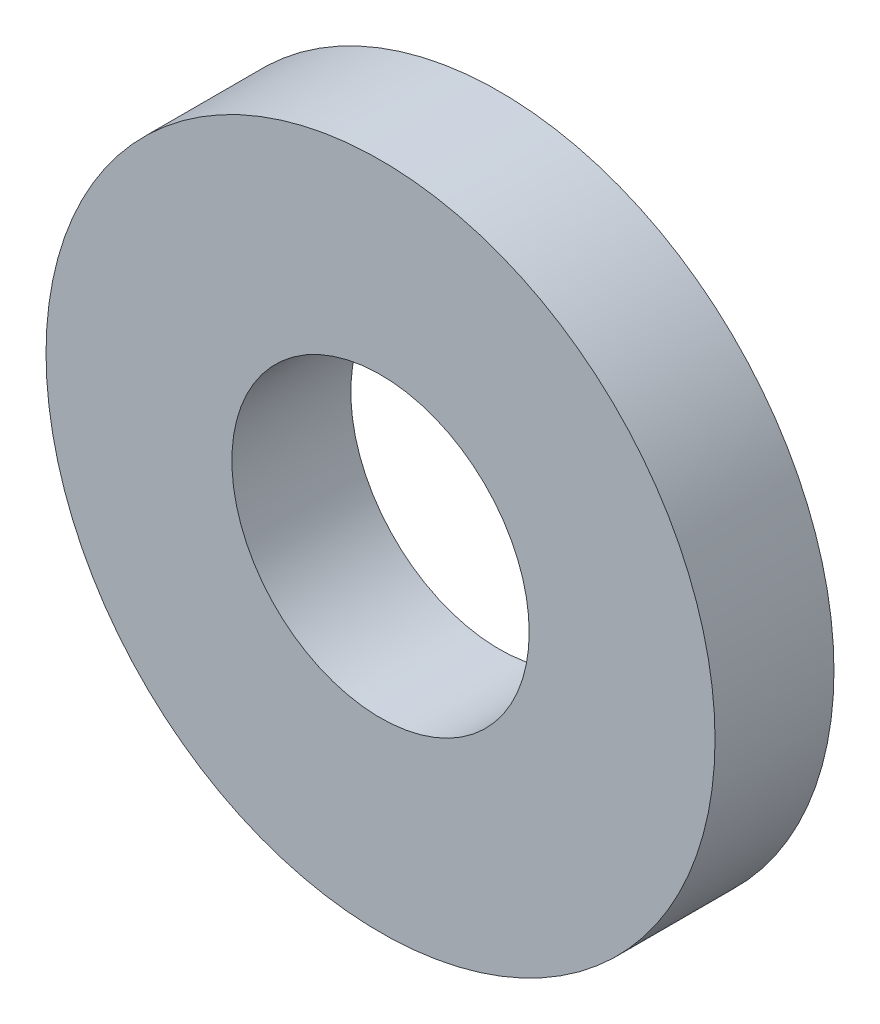
SolidWorks part; units mm, degrees
material "Plain Carbon Steel"
ref_plane "Front Plane" through (0, 0, 0) normal (0, 0, 1) x (1, 0, 0)
ref_plane "Top Plane" through (0, 0, 0) normal (0, 1, 0) x (1, 0, 0)
ref_plane "Right Plane" through (0, 0, 0) normal (1, 0, 0) x (0, 0, -1)
sketch "Washer Profile Ø45-Ø20" plane through (0, 0, 0) normal (0, 0, 1) x (1, 0, 0)
  line L0 (0, 318.1081) -> (0, -311.5066) construction
  line L2 (429.9204, 0) -> (-392.7871, 0) construction
  circle A0 centre (0, 0) radius 10
  circle A1 centre (0, 0) radius 22.5
  dimension "D1" = 20
  dimension "D2" = 45
extrude "Washer Body 8mm" add sketch "Washer Profile Ø45-Ø20" along normal blind 8
